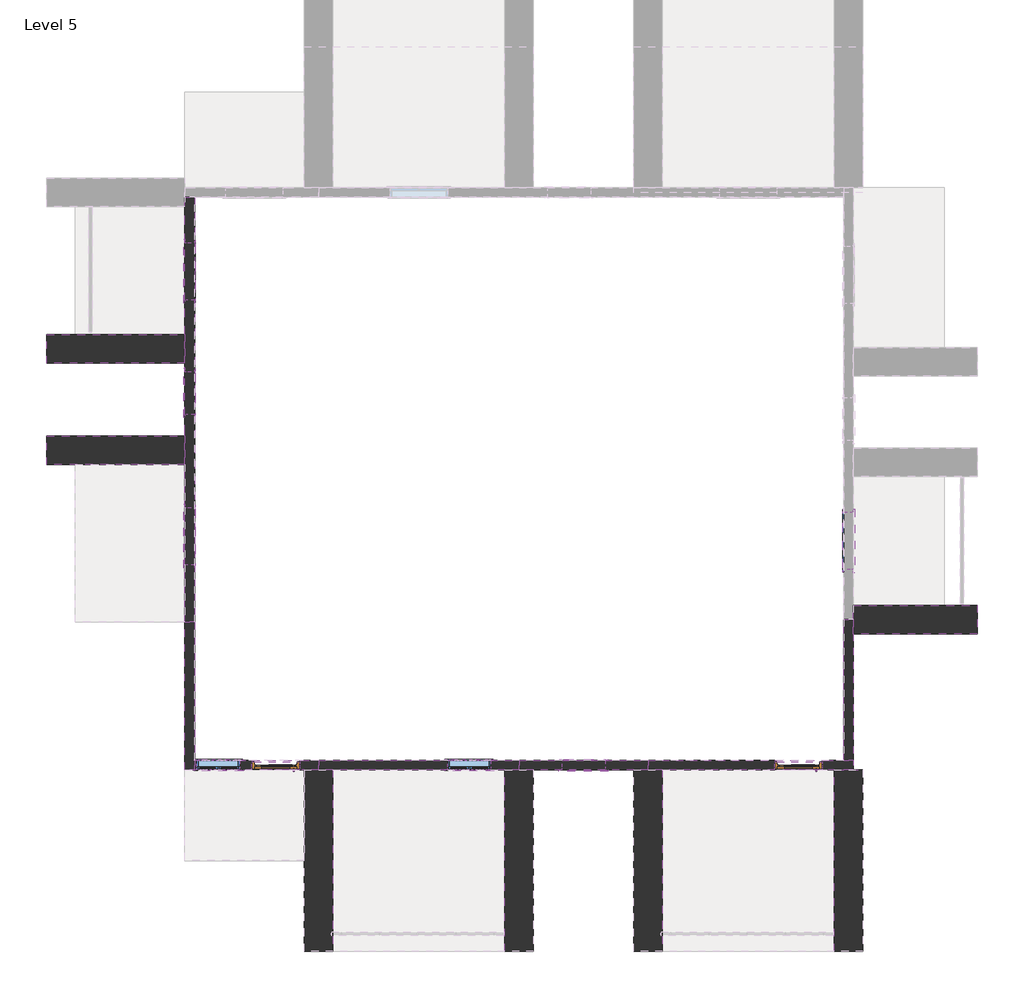
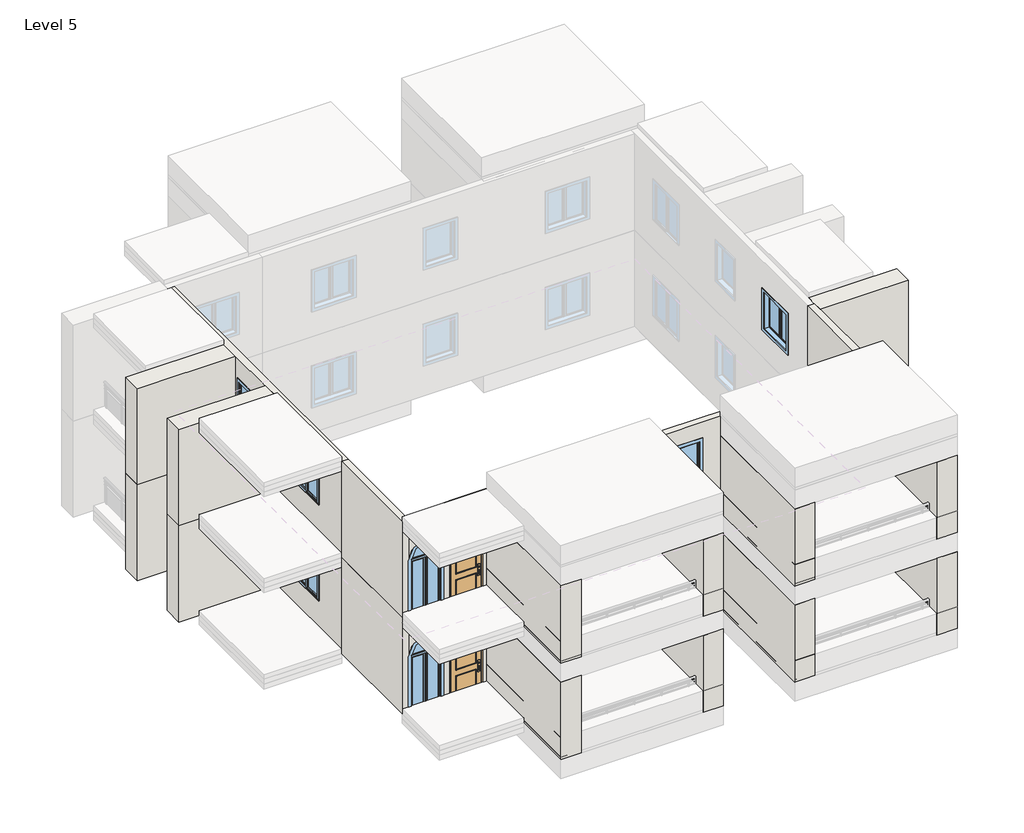
# One storey, part 1 of 4: 28 walls, 14 windows, 4 doors.
# Revit data of these elements (continued)
# Element 38 (IfcWindow, "Casement Dbl with Trim.0001 : 48\" x 48\"")
#   Mark = "50"
#   Phase Created = New Construction
#   Materials on its faces: "Sash", "Trim", "Glass"
# Element 39 (IfcWindow, "Casement Dbl with Trim.0001 : 48\" x 48\"")
#   Mark = "53"
#   Phase Created = New Construction
#   Materials on its faces: "Sash", "Trim", "Glass"
# Element 40 (IfcWindow, "Casement Dbl with Trim.0001 : 48\" x 48\"")
#   Mark = "62"
#   Phase Created = New Construction
#   Materials on its faces: "Sash", "Trim", "Glass"
# Element 41 (IfcWindow, "Casement Dbl with Trim.0001 : 48\" x 48\"")
#   Mark = "63"
#   Phase Created = New Construction
#   Materials on its faces: "Sash", "Trim", "Glass"
# Element 42 (IfcWindow, "Casement Dbl with Trim.0001 : 48\" x 48\"")
#   Mark = "66"
#   Phase Created = New Construction
#   Materials on its faces: "Sash", "Trim", "Glass"
# Element 43 (IfcWindow, "Casement with Trim : 36\" x 48\"")
#   Mark = "45"
#   Phase Created = New Construction
#   Materials on its faces: "Sash", "Trim", "Glass"
# Element 44 (IfcWindow, "Casement with Trim : 36\" x 48\"")
#   Mark = "46"
#   Phase Created = New Construction
#   Materials on its faces: "Sash", "Trim", "Glass"
# Element 45 (IfcWindow, "Casement with Trim : 36\" x 48\"")
#   Mark = "58"
#   Phase Created = New Construction
#   Materials on its faces: "Sash", "Trim", "Glass"
# Element 46 (IfcWindow, "Casement with Trim : 36\" x 48\"")
#   Mark = "59"
#   Phase Created = New Construction
#   Materials on its faces: "Sash", "Trim", "Glass"
# Materials
#   "Metal - Stainless Steel": class "Metal", colour RGB 247 247 247, transparency 0
#   "Metal - Painted - Grey": class "Paint", colour RGB 104 104 104, transparency 0
#   "Damp-proofing": class "Generic", colour RGB 127 127 127, transparency 0, Description = "Damp-proofing", Cost = 0
#   "Glass": class "Glass", colour RGB 0 128 192, transparency 0.75, Description = "Soda Lime Glass", Cost = 0
#   "Sash": class "Wood", colour RGB 224 178 126, transparency 0
#   "Trim": class "Wood", colour RGB 224 178 126, transparency 0
#   "Tile, Porcelain, 4in": class "Generic", colour RGB 89 87 158, transparency 0, Description = "Porcelain tile, 4\", white", Cost = 0
#   "Parking Stripe": class "Paint", colour RGB 250 250 91, transparency 0, Cost = 0
#   "Default Wall": colour RGB 128 128 128, transparency 0
#   "Gypsum Wall Board": class "Generic", colour RGB 127 127 127, transparency 0, Description = "Gypsum Wall Board", Cost = 0
